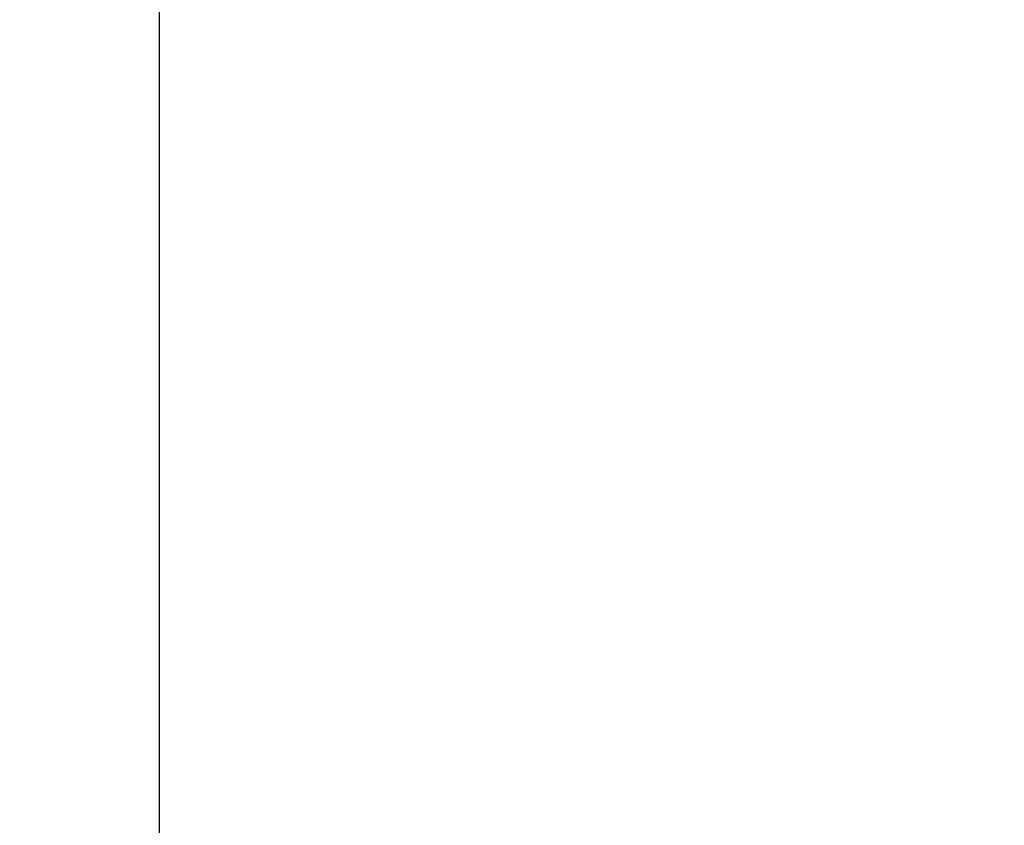
# Model space of a CAD drawing. Units: inches. Extents: x 2091 to 2899, y 967 to 2217.
# Tile 8 of 256: x 2312 to 2351, y 1032 to 1064. Entities that reach past the tile are written whole.
import ezdxf

# ---------------------------------------------------------------- set-up
doc = ezdxf.new("R2010")
doc.units = ezdxf.units.IN
doc.layers.add('A-ANNO-DIMS', color=2, linetype='Continuous', lineweight=18)
doc.styles.get("Standard").update_dxf_attribs({"font": 'arial.ttf'})
doc.dimstyles.new('ISO-25', dxfattribs={"dimtxt": 4, "dimasz": 4, "dimexe": 1.25, "dimexo": 0.625, "dimtad": 1, "dimdec": 0, "dimlunit": 3, "dimtxsty": 'Standard', "dimcen": 2.5, "dimadec": 0, "dimazin": 0, "dimtfac": 1, "dimtdec": 0, "dimtmove": 0, "dimatfit": 3, "dimfxl": 1, "dimarcsym": 0})

# ---------------------------------------------------------------- blocks, each defined once
blk = doc.blocks.new('*D68')
at = {"layer": 'A-ANNO-DIMS', "color": 0, "lineweight": -2, "transparency": 16777216}
for p, q in [((2317.144, 1535.794), (2317.144, 969.464)), ((2459.384, 1535.794), (2459.384, 969.464)), ((2321.144, 970.714), (2455.384, 970.714))]:
    blk.add_line(p, q, dxfattribs=at)
at = {"layer": 'A-ANNO-DIMS', "color": 0, "transparency": 16777216}
for points in [[(2321.144, 971.381), (2321.144, 970.048), (2317.144, 970.714)], [(2455.384, 971.381), (2455.384, 970.048), (2459.384, 970.714)]]:
    blk.add_solid(points, dxfattribs=at)
at = {"layer": 'Defpoints', "color": 0, "transparency": 16777216}
for p in [(2317.144, 1536.419), (2459.384, 1536.419), (2459.384, 970.714)]:
    blk.add_point(p, dxfattribs=at)
at = {"layer": 'A-ANNO-DIMS', "color": 0, "transparency": 16777216, "insert": (2388.264, 973.382), "char_height": 4, "attachment_point": 5}
blk.add_mtext('11\'-10"', dxfattribs=at)
blk = doc.blocks.new('*D71')
at = {"layer": 'A-ANNO-DIMS', "color": 0, "lineweight": -2, "transparency": 16777216}
for p, q in [((2212.144, 1351.294), (2212.144, 969.464)), ((2452.144, 1351.294), (2452.144, 969.464)), ((2216.144, 970.714), (2448.144, 970.714))]:
    blk.add_line(p, q, dxfattribs=at)
at = {"layer": 'A-ANNO-DIMS', "color": 0, "transparency": 16777216}
for points in [[(2216.144, 971.381), (2216.144, 970.048), (2212.144, 970.714)], [(2448.144, 971.381), (2448.144, 970.048), (2452.144, 970.714)]]:
    blk.add_solid(points, dxfattribs=at)
at = {"layer": 'Defpoints', "color": 0, "transparency": 16777216}
for p in [(2212.144, 1351.919), (2452.144, 1351.919), (2452.144, 970.714)]:
    blk.add_point(p, dxfattribs=at)
at = {"layer": 'A-ANNO-DIMS', "color": 0, "transparency": 16777216, "insert": (2332.144, 973.382), "char_height": 4, "attachment_point": 5}
blk.add_mtext('20\'-0"', dxfattribs=at)

msp = doc.modelspace()

# ---------------------------------------------------------------- dimensions: what is measured, and where the dimension line sits
at = {"layer": 'A-ANNO-DIMS'}
for base, p1, p2, picture, middle in [((2459.384, 970.714), (2317.144, 1536.419), (2459.384, 1536.419), '*D68', (2388.264, 973.382)), ((2452.144, 970.714), (2212.144, 1351.919), (2452.144, 1351.919), '*D71', (2332.144, 973.382))]:
    dim = msp.add_linear_dim(base=base, p1=p1, p2=p2, dimstyle='ISO-25', override={"dimdec": 1, "dimlfac": 1, "dimrnd": 0, "dimzin": 1, "dimdsep": 46, "dimlunit": 4, "dimfrac": 2}, dxfattribs=at)
    dim.commit()
    dim.dimension.update_dxf_attribs({"geometry": picture, "text_midpoint": middle})

doc.saveas('drawing.dxf')
